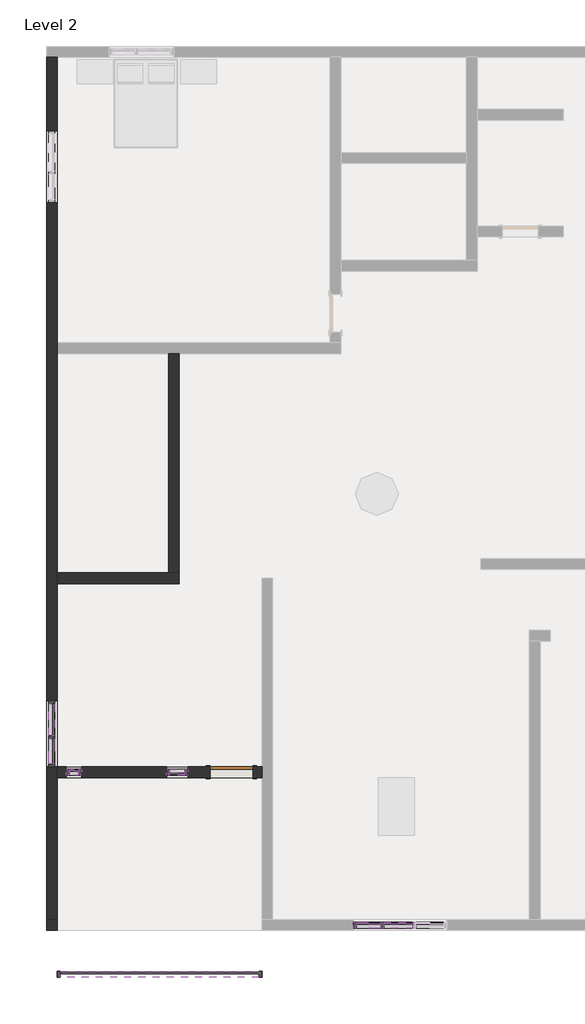
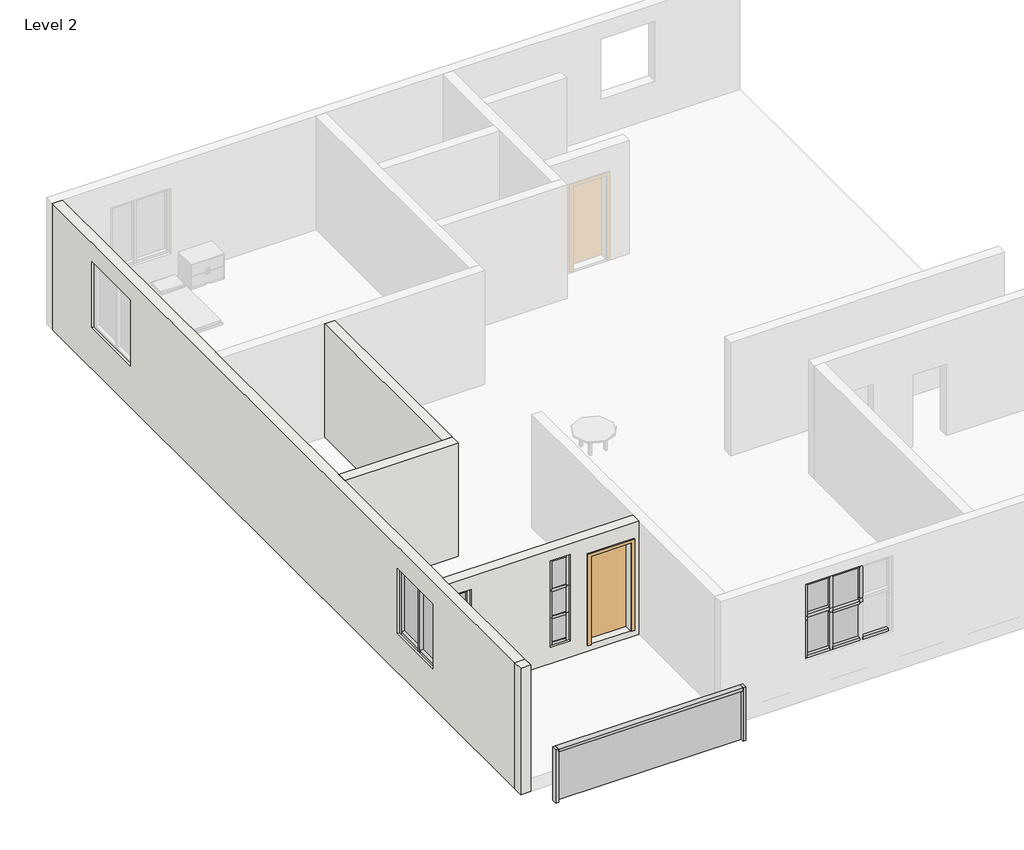
# One storey, part 1 of 3: 45 members, 13 plates, 5 walls, 1 door.
"""IFC4 building model written with IfcOpenShell, lengths in millimetres."""

from ifc_helpers import new_model, si_unit, frame, origin, place, context, project, spatial, polyline, outline, extrude, faceted_brep, transform, mapped, element, save
from components import door_0ca8825f, member_ff9f2d30, member_0c1408be, member_e5d39754, member_e31b56d3, member_3572ee78, member_a8054089, member_aa870034, member_a8964de5, member_6a93b315, member_0b7646a3, member_08dd3726, member_aaa03826, member_5b006e0e, member_fb13da3b, member_cfc5edb3, member_8ea47e38, member_081e0693, member_75a79c70, member_81de2198, member_8613ee48, member_69a5b808, member_a8c9f8c2, member_c15214c4, member_623a4a38, system_panel_glazed_ce347581, system_panel_glazed_dfb1dee4, system_panel_glazed_d46f60ed, system_panel_glazed_db16a638, system_panel_glazed_8f64e07d, system_panel_glazed_997bcd70, system_panel_glazed_706913d7, system_panel_glazed_7650606a, system_panel_glazed_1601ec89, system_panel_glazed_6c4ef35e, system_panel_glazed_6ec13f64, system_panel_glazed_f75ed1c4, system_panel_glazed_9c27a923

model = new_model("IFC4")

# Units and contexts
model_context = context("Model", 3, world=origin())
ifc_project = project(units=[si_unit("LENGTHUNIT", "METRE", prefix="MILLI")], contexts=[model_context])

# Site, building, storey
site = spatial("IfcSite", under=ifc_project)
building = spatial("IfcBuilding", under=site)
storey = spatial("IfcBuildingStorey", under=building, Name="Level 2", Elevation=3048.0)

# Door
placement = place(None, origin())
door_shape = door_0ca8825f(model_context)
element("IfcDoor", 1, ObjectType="Single-Flush : 36\" x 84\"", at=placement, inside=storey, context=model_context, shape_type="MappedRepresentation", body=[
    mapped(door_shape, transform((-15161.4702714, -8234.9383903, 3505.2), x_axis=(1.0, 0.0, 0.0), y_axis=(0.0, 1.0, 0.0), z_axis=(0.0, 0.0, 1.0))),
])

# Members
member_shape = member_ff9f2d30(model_context)
element("IfcMember", 2, ObjectType="Rectangular Mullion : 2.5\" x 5\" rectangular", at=placement, inside=storey, context=model_context, shape_type="MappedRepresentation", body=[
    mapped(member_shape, transform((-16469.5702714, -8234.9383903, 5829.1309578), x_axis=(0.0, 0.0, 1.0), y_axis=(0.0, 1.0, 0.0), z_axis=(-1.0, 0.0, 0.0))),
])
element("IfcMember", 3, ObjectType="Rectangular Mullion : 2.5\" x 5\" rectangular", at=placement, inside=storey, context=model_context, shape_type="MappedRepresentation", body=[
    mapped(member_shape, transform((-16139.3702714, -8234.9383903, 3746.1211233), x_axis=(0.0, 0.0, -1.0), y_axis=(0.0, 1.0, 0.0), z_axis=(1.0, 0.0, 0.0))),
])
member_2_shape = member_0c1408be(model_context)
element("IfcMember", 4, ObjectType="Rectangular Mullion : 2.5\" x 5\" rectangular", at=placement, inside=storey, context=model_context, shape_type="MappedRepresentation", body=[
    mapped(member_2_shape, transform((-16469.5702714, -8234.9383903, 5067.1309578), x_axis=(0.0, 0.0, 1.0), y_axis=(0.0, 1.0, 0.0), z_axis=(-1.0, 0.0, 0.0))),
])
element("IfcMember", 5, ObjectType="Rectangular Mullion : 2.5\" x 5\" rectangular", at=placement, inside=storey, context=model_context, shape_type="MappedRepresentation", body=[
    mapped(member_2_shape, transform((-16469.5702714, -8234.9383903, 4406.6260406), x_axis=(0.0, 0.0, 1.0), y_axis=(0.0, 1.0, 0.0), z_axis=(-1.0, 0.0, 0.0))),
])
member_3_shape = member_e5d39754(model_context)
element("IfcMember", 6, ObjectType="Rectangular Mullion : 2.5\" x 5\" rectangular", at=placement, inside=storey, context=model_context, shape_type="MappedRepresentation", body=[
    mapped(member_3_shape, transform((-11243.5202714, -11473.4383903, 4012.7558847), x_axis=(0.0, 0.0, -1.0), y_axis=(0.0, -1.0, 0.0), z_axis=(-1.0, 0.0, 0.0))),
])
member_4_shape = member_e31b56d3(model_context)
element("IfcMember", 7, ObjectType="Rectangular Mullion : 2.5\" x 5\" rectangular", at=placement, inside=storey, context=model_context, shape_type="MappedRepresentation", body=[
    mapped(member_4_shape, transform((-18666.6702714, -8234.9383903, 5016.6712267), x_axis=(-1.0, 0.0, 0.0), y_axis=(0.0, -1.0, 0.0), z_axis=(0.0, 0.0, 1.0))),
])
element("IfcMember", 8, ObjectType="Rectangular Mullion : 2.5\" x 5\" rectangular", at=placement, inside=storey, context=model_context, shape_type="MappedRepresentation", body=[
    mapped(member_4_shape, transform((-18666.6702714, -8234.9383903, 4376.9636561), x_axis=(-1.0, 0.0, 0.0), y_axis=(0.0, -1.0, 0.0), z_axis=(0.0, 0.0, 1.0))),
])
member_5_shape = member_3572ee78(model_context)
element("IfcMember", 9, ObjectType="Rectangular Mullion : 2.5\" x 5\" rectangular", at=placement, inside=storey, context=model_context, shape_type="MappedRepresentation", body=[
    mapped(member_5_shape, transform((-18399.9702714, -8234.9383903, 5016.6712267), x_axis=(0.0, 0.0, 1.0), y_axis=(0.0, -1.0, 0.0), z_axis=(1.0, 0.0, 0.0))),
])
element("IfcMember", 10, ObjectType="Rectangular Mullion : 2.5\" x 5\" rectangular", at=placement, inside=storey, context=model_context, shape_type="MappedRepresentation", body=[
    mapped(member_5_shape, transform((-18399.9702714, -8234.9383903, 4376.9636561), x_axis=(0.0, 0.0, 1.0), y_axis=(0.0, -1.0, 0.0), z_axis=(1.0, 0.0, 0.0))),
])
member_6_shape = member_a8054089(model_context)
element("IfcMember", 11, ObjectType="Rectangular Mullion : 2.5\" x 5\" rectangular", at=placement, inside=storey, context=model_context, shape_type="MappedRepresentation", body=[
    mapped(member_6_shape, transform((-18603.1702714, -8234.9383903, 3737.2560855), x_axis=(0.0, 0.0, -1.0), y_axis=(0.0, -1.0, 0.0), z_axis=(-1.0, 0.0, 0.0))),
])
element("IfcMember", 12, ObjectType="Rectangular Mullion : 2.5\" x 5\" rectangular", at=placement, inside=storey, context=model_context, shape_type="MappedRepresentation", body=[
    mapped(member_4_shape, transform((-18336.4702714, -8234.9383903, 4376.9636561), x_axis=(1.0, 0.0, 0.0), y_axis=(0.0, -1.0, 0.0), z_axis=(0.0, 0.0, -1.0))),
])
element("IfcMember", 13, ObjectType="Rectangular Mullion : 2.5\" x 5\" rectangular", at=placement, inside=storey, context=model_context, shape_type="MappedRepresentation", body=[
    mapped(member_4_shape, transform((-18336.4702714, -8234.9383903, 3737.2560855), x_axis=(1.0, 0.0, 0.0), y_axis=(0.0, -1.0, 0.0), z_axis=(0.0, 0.0, -1.0))),
])
element("IfcMember", 14, ObjectType="Rectangular Mullion : 2.5\" x 5\" rectangular", at=placement, inside=storey, context=model_context, shape_type="MappedRepresentation", body=[
    mapped(member_6_shape, transform((-18399.9702714, -8234.9383903, 5778.6712267), x_axis=(0.0, 0.0, 1.0), y_axis=(0.0, -1.0, 0.0), z_axis=(1.0, 0.0, 0.0))),
])
member_7_shape = member_aa870034(model_context)
element("IfcMember", 15, ObjectType="Rectangular Mullion : 2.5\" x 5\" rectangular", at=placement, inside=storey, context=model_context, shape_type="MappedRepresentation", body=[
    mapped(member_7_shape, transform((-18666.6702714, -8234.9383903, 5778.6712267), x_axis=(-1.0, 0.0, 0.0), y_axis=(0.0, -1.0, 0.0), z_axis=(0.0, 0.0, 1.0))),
])
element("IfcMember", 16, ObjectType="Rectangular Mullion : 2.5\" x 5\" rectangular", at=placement, inside=storey, context=model_context, shape_type="MappedRepresentation", body=[
    mapped(member_7_shape, transform((-16075.8702714, -8234.9383903, 5829.1309578), x_axis=(1.0, 0.0, 0.0), y_axis=(0.0, 1.0, 0.0), z_axis=(0.0, 0.0, 1.0))),
])
element("IfcMember", 17, ObjectType="Rectangular Mullion : 2.5\" x 5\" rectangular", at=placement, inside=storey, context=model_context, shape_type="MappedRepresentation", body=[
    mapped(member_7_shape, transform((-18336.4702714, -8234.9383903, 5016.6712267), x_axis=(1.0, 0.0, 0.0), y_axis=(0.0, -1.0, 0.0), z_axis=(0.0, 0.0, -1.0))),
])
element("IfcMember", 18, ObjectType="Rectangular Mullion : 2.5\" x 5\" rectangular", at=placement, inside=storey, context=model_context, shape_type="MappedRepresentation", body=[
    mapped(member_7_shape, transform((-16533.0702714, -8234.9383903, 5067.1309578), x_axis=(-1.0, 0.0, 0.0), y_axis=(0.0, 1.0, 0.0), z_axis=(0.0, 0.0, -1.0))),
])
member_8_shape = member_a8964de5(model_context)
element("IfcMember", 19, ObjectType="Rectangular Mullion : 2.5\" x 5\" rectangular", at=placement, inside=storey, context=model_context, shape_type="MappedRepresentation", body=[
    mapped(member_8_shape, transform((-16533.0702714, -8234.9383903, 4406.6260406), x_axis=(-1.0, 0.0, 0.0), y_axis=(0.0, 1.0, 0.0), z_axis=(0.0, 0.0, -1.0))),
])
element("IfcMember", 20, ObjectType="Rectangular Mullion : 2.5\" x 5\" rectangular", at=placement, inside=storey, context=model_context, shape_type="MappedRepresentation", body=[
    mapped(member_8_shape, transform((-16075.8702714, -8234.9383903, 5067.1309578), x_axis=(1.0, 0.0, 0.0), y_axis=(0.0, 1.0, 0.0), z_axis=(0.0, 0.0, 1.0))),
])
element("IfcMember", 21, ObjectType="Rectangular Mullion : 2.5\" x 5\" rectangular", at=placement, inside=storey, context=model_context, shape_type="MappedRepresentation", body=[
    mapped(member_8_shape, transform((-16533.0702714, -8234.9383903, 3746.1211233), x_axis=(-1.0, 0.0, 0.0), y_axis=(0.0, 1.0, 0.0), z_axis=(0.0, 0.0, -1.0))),
])
element("IfcMember", 22, ObjectType="Rectangular Mullion : 2.5\" x 5\" rectangular", at=placement, inside=storey, context=model_context, shape_type="MappedRepresentation", body=[
    mapped(member_8_shape, transform((-16075.8702714, -8234.9383903, 4406.6260406), x_axis=(1.0, 0.0, 0.0), y_axis=(0.0, 1.0, 0.0), z_axis=(0.0, 0.0, 1.0))),
])
member_9_shape = member_6a93b315(model_context)
element("IfcMember", 23, ObjectType="Rectangular Mullion : 2.5\" x 5\" rectangular", at=placement, inside=storey, context=model_context, shape_type="MappedRepresentation", body=[
    mapped(member_9_shape, transform((-12570.6702714, -11473.4383903, 4928.9320171), x_axis=(-1.0, 0.0, 0.0), y_axis=(0.0, -1.0, 0.0), z_axis=(0.0, 0.0, 1.0))),
])
member_10_shape = member_0b7646a3(model_context)
element("IfcMember", 24, ObjectType="Rectangular Mullion : 2.5\" x 5\" rectangular", at=placement, inside=storey, context=model_context, shape_type="MappedRepresentation", body=[
    mapped(member_10_shape, transform((-11992.8202714, -11473.4383903, 5845.1081495), x_axis=(0.0, 0.0, 1.0), y_axis=(0.0, -1.0, 0.0), z_axis=(1.0, 0.0, 0.0))),
])
element("IfcMember", 25, ObjectType="Rectangular Mullion : 2.5\" x 5\" rectangular", at=placement, inside=storey, context=model_context, shape_type="MappedRepresentation", body=[
    mapped(member_10_shape, transform((-12507.1702714, -11473.4383903, 4012.7558847), x_axis=(0.0, 0.0, -1.0), y_axis=(0.0, -1.0, 0.0), z_axis=(-1.0, 0.0, 0.0))),
])
member_11_shape = member_08dd3726(model_context)
element("IfcMember", 26, ObjectType="Rectangular Mullion : 2.5\" x 5\" rectangular", at=placement, inside=storey, context=model_context, shape_type="MappedRepresentation", body=[
    mapped(member_11_shape, transform((-11961.0702714, -11473.4383903, 5030.5320171), x_axis=(1.0, 0.0, 0.0), y_axis=(0.0, -1.0, 0.0), z_axis=(0.0, 0.0, -1.0))),
])
element("IfcMember", 27, ObjectType="Rectangular Mullion : 2.5\" x 5\" rectangular", at=placement, inside=storey, context=model_context, shape_type="MappedRepresentation", body=[
    mapped(member_11_shape, transform((-11275.2702714, -11473.4383903, 5030.5320171), x_axis=(1.0, 0.0, 0.0), y_axis=(0.0, -1.0, 0.0), z_axis=(0.0, 0.0, -1.0))),
])
member_12_shape = member_aaa03826(model_context)
element("IfcMember", 28, ObjectType="Rectangular Mullion : 2.5\" x 5\" rectangular", at=placement, inside=storey, context=model_context, shape_type="MappedRepresentation", body=[
    mapped(member_12_shape, transform((-11992.8202714, -11473.4383903, 5030.5320171), x_axis=(0.0, 0.0, 1.0), y_axis=(0.0, -1.0, 0.0), z_axis=(1.0, 0.0, 0.0))),
])
member_13_shape = member_5b006e0e(model_context)
element("IfcMember", 29, ObjectType="Rectangular Mullion : 2.5\" x 5\" rectangular", at=placement, inside=storey, context=model_context, shape_type="MappedRepresentation", body=[
    mapped(member_13_shape, transform((-12570.6702714, -11473.4383903, 5845.1081495), x_axis=(-1.0, 0.0, 0.0), y_axis=(0.0, -1.0, 0.0), z_axis=(0.0, 0.0, 1.0))),
])
member_14_shape = member_fb13da3b(model_context)
element("IfcMember", 30, ObjectType="Rectangular Mullion : 2.5\" x 5\" rectangular", at=placement, inside=storey, context=model_context, shape_type="MappedRepresentation", body=[
    mapped(member_14_shape, transform((-12570.6702714, -11473.4383903, 5030.5320171), x_axis=(-1.0, 0.0, 0.0), y_axis=(0.0, -1.0, 0.0), z_axis=(0.0, 0.0, 1.0))),
])
member_15_shape = member_cfc5edb3(model_context)
element("IfcMember", 31, ObjectType="Rectangular Mullion : 2.5\" x 5\" rectangular", at=placement, inside=storey, context=model_context, shape_type="MappedRepresentation", body=[
    mapped(member_15_shape, transform((-11961.0702714, -11473.4383903, 4928.9320171), x_axis=(1.0, 0.0, 0.0), y_axis=(0.0, -1.0, 0.0), z_axis=(0.0, 0.0, -1.0))),
])
element("IfcMember", 32, ObjectType="Rectangular Mullion : 2.5\" x 5\" rectangular", at=placement, inside=storey, context=model_context, shape_type="MappedRepresentation", body=[
    mapped(member_15_shape, transform((-11275.2702714, -11473.4383903, 4928.9320171), x_axis=(1.0, 0.0, 0.0), y_axis=(0.0, -1.0, 0.0), z_axis=(0.0, 0.0, -1.0))),
])
member_16_shape = member_8ea47e38(model_context)
element("IfcMember", 33, ObjectType="Rectangular Mullion : 2.5\" x 5\" rectangular", at=placement, inside=storey, context=model_context, shape_type="MappedRepresentation", body=[
    mapped(member_16_shape, transform((-11961.0702714, -11473.4383903, 4012.7558847), x_axis=(1.0, 0.0, 0.0), y_axis=(0.0, -1.0, 0.0), z_axis=(0.0, 0.0, -1.0))),
])
member_17_shape = member_081e0693(model_context)
element("IfcMember", 34, ObjectType="Rectangular Mullion : 2.5\" x 5\" rectangular", at=placement, inside=storey, context=model_context, shape_type="MappedRepresentation", body=[
    mapped(member_17_shape, transform((-11929.3202714, -11473.4383903, 4012.7558847), x_axis=(0.0, 0.0, -1.0), y_axis=(0.0, -1.0, 0.0), z_axis=(-1.0, 0.0, 0.0))),
])
element("IfcMember", 35, ObjectType="Rectangular Mullion : 2.5\" x 5\" rectangular", at=placement, inside=storey, context=model_context, shape_type="MappedRepresentation", body=[
    mapped(member_17_shape, transform((-11307.0202714, -11473.4383903, 5845.1081495), x_axis=(0.0, 0.0, 1.0), y_axis=(0.0, -1.0, 0.0), z_axis=(1.0, 0.0, 0.0))),
])
member_18_shape = member_75a79c70(model_context)
element("IfcMember", 36, ObjectType="Rectangular Mullion : 2.5\" x 5\" rectangular", at=placement, inside=storey, context=model_context, shape_type="MappedRepresentation", body=[
    mapped(member_18_shape, transform((-11307.0202714, -11473.4383903, 4928.9320171), x_axis=(0.0, 0.0, 1.0), y_axis=(0.0, -1.0, 0.0), z_axis=(1.0, 0.0, 0.0))),
])
member_19_shape = member_81de2198(model_context)
element("IfcMember", 37, ObjectType="Rectangular Mullion : 2.5\" x 5\" rectangular", at=placement, inside=storey, context=model_context, shape_type="MappedRepresentation", body=[
    mapped(member_19_shape, transform((-18971.4702714, -8057.1383903, 5555.3141516), x_axis=(0.0, 0.0, 1.0), y_axis=(-1.0, 0.0, 0.0), z_axis=(0.0, -1.0, 0.0))),
])
element("IfcMember", 38, ObjectType="Rectangular Mullion : 2.5\" x 5\" rectangular", at=placement, inside=storey, context=model_context, shape_type="MappedRepresentation", body=[
    mapped(member_19_shape, transform((-18971.4702714, -7517.3883903, 3979.8466642), x_axis=(0.0, 0.0, -1.0), y_axis=(-1.0, 0.0, 0.0), z_axis=(0.0, 1.0, 0.0))),
])
member_20_shape = member_8613ee48(model_context)
element("IfcMember", 39, ObjectType="Rectangular Mullion : 2.5\" x 5\" rectangular", at=placement, inside=storey, context=model_context, shape_type="MappedRepresentation", body=[
    mapped(member_20_shape, transform((-18971.4702714, -7453.8883903, 5555.3141516), x_axis=(0.0, 0.0, 1.0), y_axis=(-1.0, 0.0, 0.0), z_axis=(0.0, -1.0, 0.0))),
])
member_21_shape = member_69a5b808(model_context)
element("IfcMember", 40, ObjectType="Rectangular Mullion : 2.5\" x 5\" rectangular", at=placement, inside=storey, context=model_context, shape_type="MappedRepresentation", body=[
    mapped(member_21_shape, transform((-18971.4702714, -7485.6383903, 3979.8466642), x_axis=(0.0, -1.0, 0.0), y_axis=(-1.0, 0.0, 0.0), z_axis=(0.0, 0.0, -1.0))),
])
element("IfcMember", 41, ObjectType="Rectangular Mullion : 2.5\" x 5\" rectangular", at=placement, inside=storey, context=model_context, shape_type="MappedRepresentation", body=[
    mapped(member_20_shape, transform((-18971.4702714, -6774.4383903, 3979.8466642), x_axis=(0.0, 0.0, -1.0), y_axis=(-1.0, 0.0, 0.0), z_axis=(0.0, 1.0, 0.0))),
])
member_22_shape = member_a8c9f8c2(model_context)
element("IfcMember", 42, ObjectType="Rectangular Mullion : 2.5\" x 5\" rectangular", at=placement, inside=storey, context=model_context, shape_type="MappedRepresentation", body=[
    mapped(member_22_shape, transform((-18971.4702714, -6710.9383903, 5555.3141516), x_axis=(0.0, 1.0, 0.0), y_axis=(-1.0, 0.0, 0.0), z_axis=(0.0, 0.0, 1.0))),
])
element("IfcMember", 43, ObjectType="Rectangular Mullion : 2.5\" x 5\" rectangular", at=placement, inside=storey, context=model_context, shape_type="MappedRepresentation", body=[
    mapped(member_22_shape, transform((-18971.4702714, -8120.6383903, 3979.8466642), x_axis=(0.0, -1.0, 0.0), y_axis=(-1.0, 0.0, 0.0), z_axis=(0.0, 0.0, -1.0))),
])
member_23_shape = member_c15214c4(model_context)
element("IfcMember", 44, ObjectType="Rectangular Mullion : 2.5\" x 5\" rectangular", at=placement, inside=storey, context=model_context, shape_type="MappedRepresentation", body=[
    mapped(member_23_shape, transform((-18857.1702714, -12520.0349955, 4647.0701096), x_axis=(-1.0, 0.0, 0.0), y_axis=(0.0, -1.0, 0.0), z_axis=(0.0, 0.0, 1.0))),
])
member_24_shape = member_623a4a38(model_context)
element("IfcMember", 45, ObjectType="Rectangular Mullion : 2.5\" x 5\" rectangular", at=placement, inside=storey, context=model_context, shape_type="MappedRepresentation", body=[
    mapped(member_24_shape, transform((-14577.2702714, -12520.0349955, 4647.0701096), x_axis=(0.0, 0.0, 1.0), y_axis=(0.0, -1.0, 0.0), z_axis=(1.0, 0.0, 0.0))),
])
element("IfcMember", 46, ObjectType="Rectangular Mullion : 2.5\" x 5\" rectangular", at=placement, inside=storey, context=model_context, shape_type="MappedRepresentation", body=[
    mapped(member_23_shape, transform((-14513.7702714, -12520.0349955, 3361.4365062), x_axis=(1.0, 0.0, 0.0), y_axis=(0.0, -1.0, 0.0), z_axis=(0.0, 0.0, -1.0))),
])

# Plates
system_panel_glazed_shape = system_panel_glazed_ce347581(model_context)
element("IfcPlate", 47, ObjectType="System Panel : Glazed", at=placement, inside=storey, context=model_context, shape_type="MappedRepresentation", body=[
    mapped(system_panel_glazed_shape, transform((-18501.5702714, -8234.9383903, 3800.7560855), x_axis=(1.0, 0.0, 0.0), y_axis=(0.0, 1.0, 0.0), z_axis=(0.0, 0.0, 1.0))),
])
system_panel_glazed_2_shape = system_panel_glazed_dfb1dee4(model_context)
element("IfcPlate", 48, ObjectType="System Panel : Glazed", at=placement, inside=storey, context=model_context, shape_type="MappedRepresentation", body=[
    mapped(system_panel_glazed_2_shape, transform((-18501.5702714, -8234.9383903, 4408.7136561), x_axis=(1.0, 0.0, 0.0), y_axis=(0.0, 1.0, 0.0), z_axis=(0.0, 0.0, 1.0))),
])
system_panel_glazed_3_shape = system_panel_glazed_d46f60ed(model_context)
element("IfcPlate", 49, ObjectType="System Panel : Glazed", at=placement, inside=storey, context=model_context, shape_type="MappedRepresentation", body=[
    mapped(system_panel_glazed_3_shape, transform((-18501.5702714, -8234.9383903, 5048.4212267), x_axis=(1.0, 0.0, 0.0), y_axis=(0.0, 1.0, 0.0), z_axis=(0.0, 0.0, 1.0))),
])
system_panel_glazed_4_shape = system_panel_glazed_db16a638(model_context)
element("IfcPlate", 50, ObjectType="System Panel : Glazed", at=placement, inside=storey, context=model_context, shape_type="MappedRepresentation", body=[
    mapped(system_panel_glazed_4_shape, transform((-16304.4702714, -8234.9383903, 5098.8809578), x_axis=(-1.0, 0.0, 0.0), y_axis=(0.0, -1.0, 0.0), z_axis=(0.0, 0.0, 1.0))),
])
system_panel_glazed_5_shape = system_panel_glazed_8f64e07d(model_context)
element("IfcPlate", 51, ObjectType="System Panel : Glazed", at=placement, inside=storey, context=model_context, shape_type="MappedRepresentation", body=[
    mapped(system_panel_glazed_5_shape, transform((-16304.4702714, -8234.9383903, 4438.3760406), x_axis=(-1.0, 0.0, 0.0), y_axis=(0.0, -1.0, 0.0), z_axis=(0.0, 0.0, 1.0))),
])
system_panel_glazed_6_shape = system_panel_glazed_997bcd70(model_context)
element("IfcPlate", 52, ObjectType="System Panel : Glazed", at=placement, inside=storey, context=model_context, shape_type="MappedRepresentation", body=[
    mapped(system_panel_glazed_6_shape, transform((-16304.4702714, -8234.9383903, 3809.6211233), x_axis=(-1.0, 0.0, 0.0), y_axis=(0.0, -1.0, 0.0), z_axis=(0.0, 0.0, 1.0))),
])
system_panel_glazed_7_shape = system_panel_glazed_706913d7(model_context)
element("IfcPlate", 53, ObjectType="System Panel : Glazed", at=placement, inside=storey, context=model_context, shape_type="MappedRepresentation", body=[
    mapped(system_panel_glazed_7_shape, transform((-12249.9952714, -11473.4383903, 4076.2558847), x_axis=(1.0, 0.0, 0.0), y_axis=(0.0, 1.0, 0.0), z_axis=(0.0, 0.0, 1.0))),
])
system_panel_glazed_8_shape = system_panel_glazed_7650606a(model_context)
element("IfcPlate", 54, ObjectType="System Panel : Glazed", at=placement, inside=storey, context=model_context, shape_type="MappedRepresentation", body=[
    mapped(system_panel_glazed_8_shape, transform((-12249.9952714, -11473.4383903, 5062.2820171), x_axis=(1.0, 0.0, 0.0), y_axis=(0.0, 1.0, 0.0), z_axis=(0.0, 0.0, 1.0))),
])
system_panel_glazed_9_shape = system_panel_glazed_1601ec89(model_context)
element("IfcPlate", 55, ObjectType="System Panel : Glazed", at=placement, inside=storey, context=model_context, shape_type="MappedRepresentation", body=[
    mapped(system_panel_glazed_9_shape, transform((-11618.1702714, -11473.4383903, 4076.2558847), x_axis=(1.0, 0.0, 0.0), y_axis=(0.0, 1.0, 0.0), z_axis=(0.0, 0.0, 1.0))),
])
system_panel_glazed_10_shape = system_panel_glazed_6c4ef35e(model_context)
element("IfcPlate", 56, ObjectType="System Panel : Glazed", at=placement, inside=storey, context=model_context, shape_type="MappedRepresentation", body=[
    mapped(system_panel_glazed_10_shape, transform((-11618.1702714, -11473.4383903, 4960.6820171), x_axis=(1.0, 0.0, 0.0), y_axis=(0.0, 1.0, 0.0), z_axis=(0.0, 0.0, 1.0))),
])
system_panel_glazed_11_shape = system_panel_glazed_6ec13f64(model_context)
element("IfcPlate", 57, ObjectType="System Panel : Glazed", at=placement, inside=storey, context=model_context, shape_type="MappedRepresentation", body=[
    mapped(system_panel_glazed_11_shape, transform((-18971.4702714, -7114.1633903, 4043.3466642), x_axis=(0.0, -1.0, 0.0), y_axis=(1.0, 0.0, 0.0), z_axis=(0.0, 0.0, 1.0))),
])
system_panel_glazed_12_shape = system_panel_glazed_f75ed1c4(model_context)
element("IfcPlate", 58, ObjectType="System Panel : Glazed", at=placement, inside=storey, context=model_context, shape_type="MappedRepresentation", body=[
    mapped(system_panel_glazed_12_shape, transform((-18971.4702714, -7787.2633903, 4043.3466642), x_axis=(0.0, -1.0, 0.0), y_axis=(1.0, 0.0, 0.0), z_axis=(0.0, 0.0, 1.0))),
])
system_panel_glazed_13_shape = system_panel_glazed_9c27a923(model_context)
element("IfcPlate", 59, ObjectType="System Panel : Glazed", at=placement, inside=storey, context=model_context, shape_type="MappedRepresentation", body=[
    mapped(system_panel_glazed_13_shape, transform((-16685.4702714, -12520.0349955, 3361.4365062), x_axis=(1.0, 0.0, 0.0), y_axis=(0.0, 1.0, 0.0), z_axis=(0.0, 0.0, 1.0))),
])

# Walls
element("IfcWall", 60, ObjectType="9\"", at=placement, inside=storey, context=model_context, shape_type="Brep", body=[
    faceted_brep([(-19085.7702714, 6928.8616097, 3048.0), (-19085.7702714, -11359.1383903, 3048.0), (-19085.7702714, -11359.1383903, 6096.0), (-19085.7702714, 6928.8616097, 6096.0), (-19085.7702714, 5366.7616097, 4041.7365925), (-19085.7702714, 5366.7616097, 5636.3811186), (-19085.7702714, 3842.7616097, 5636.3811186), (-19085.7702714, 3842.7616097, 4041.7365925), (-19085.7702714, -6710.9383903, 3979.8466642), (-19085.7702714, -6710.9383903, 5555.3141516), (-19085.7702714, -8120.6383903, 5555.3141516), (-19085.7702714, -8120.6383903, 3979.8466642), (-18857.1702714, -11359.1383903, 3048.0), (-18857.1702714, -8349.2383903, 3048.0), (-18857.1702714, -8120.6383903, 3048.0), (-18857.1702714, -4234.4383903, 3048.0), (-18857.1702714, -4005.8383903, 3048.0), (-18857.1702714, 642.3616097, 3048.0), (-18857.1702714, 870.9616097, 3048.0), (-18857.1702714, 6928.8616097, 3048.0), (-18857.1702714, 6928.8616097, 6096.0), (-18857.1702714, 870.9616097, 6096.0), (-18857.1702714, 642.3616097, 6096.0), (-18857.1702714, -4005.8383903, 6096.0), (-18857.1702714, -4234.4383903, 6096.0), (-18857.1702714, -8120.6383903, 6096.0), (-18857.1702714, -8349.2383903, 6096.0), (-18857.1702714, -11359.1383903, 6096.0), (-18857.1702714, 5366.7616097, 5636.3811186), (-18857.1702714, 5366.7616097, 4041.7365925), (-18857.1702714, 3842.7616097, 4041.7365925), (-18857.1702714, 3842.7616097, 5636.3811186), (-18857.1702714, -6710.9383903, 5555.3141516), (-18857.1702714, -6710.9383903, 3979.8466642), (-18857.1702714, -8120.6383903, 3979.8466642), (-18857.1702714, -8120.6383903, 5555.3141516)], [[[0, 1, 2, 3], [4, 5, 6, 7], [8, 9, 10, 11]], [[12, 13, 14, 15, 16, 17, 18, 19, 20, 21, 22, 23, 24, 25, 26, 27], [28, 29, 30, 31], [32, 33, 34, 35]], [[1, 0, 19, 18, 17, 16, 15, 14, 13, 12]], [[3, 2, 27, 26, 25, 24, 23, 22, 21, 20]], [[0, 3, 20, 19]], [[2, 1, 12, 27]], [[28, 5, 4, 29]], [[5, 28, 31, 6]], [[6, 31, 30, 7]], [[29, 4, 7, 30]], [[8, 33, 32, 9]], [[9, 32, 35, 10]], [[10, 35, 34, 11]], [[33, 8, 11, 34]]]),
])
element("IfcWall", 61, ObjectType="9\"", at=placement, inside=storey, context=model_context, shape_type="Brep", body=[
    faceted_brep([(-18857.1702714, -8349.2383903, 3048.0), (-14513.7702714, -8349.2383903, 3048.0), (-14513.7702714, -8349.2383903, 6096.0), (-18857.1702714, -8349.2383903, 6096.0), (-18666.6702714, -8349.2383903, 3737.2560855), (-18666.6702714, -8349.2383903, 5778.6712267), (-18336.4702714, -8349.2383903, 5778.6712267), (-18336.4702714, -8349.2383903, 3737.2560855), (-15618.6702714, -8349.2383903, 3505.2), (-15618.6702714, -8349.2383903, 5638.8), (-14704.2702714, -8349.2383903, 5638.8), (-14704.2702714, -8349.2383903, 3505.2), (-16075.8702714, -8349.2383903, 5829.1309578), (-16075.8702714, -8349.2383903, 3746.1211233), (-16533.0702714, -8349.2383903, 3746.1211233), (-16533.0702714, -8349.2383903, 5829.1309578), (-14513.7702714, -8120.6383903, 3048.0), (-18857.1702714, -8120.6383903, 3048.0), (-18857.1702714, -8120.6383903, 3979.8466642), (-18857.1702714, -8120.6383903, 5555.3141516), (-18857.1702714, -8120.6383903, 6096.0), (-14513.7702714, -8120.6383903, 6096.0), (-18666.6702714, -8120.6383903, 5778.6712267), (-18666.6702714, -8120.6383903, 3737.2560855), (-18336.4702714, -8120.6383903, 3737.2560855), (-18336.4702714, -8120.6383903, 5778.6712267), (-15618.6702714, -8120.6383903, 3505.2), (-14704.2702714, -8120.6383903, 3505.2), (-14704.2702714, -8120.6383903, 5638.8), (-15618.6702714, -8120.6383903, 5638.8), (-16075.8702714, -8120.6383903, 3746.1211233), (-16075.8702714, -8120.6383903, 5829.1309578), (-16533.0702714, -8120.6383903, 5829.1309578), (-16533.0702714, -8120.6383903, 3746.1211233)], [[[0, 1, 2, 3], [4, 5, 6, 7], [8, 9, 10, 11], [12, 13, 14, 15]], [[16, 17, 18, 19, 20, 21], [22, 23, 24, 25], [26, 27, 28, 29], [30, 31, 32, 33]], [[1, 0, 17, 16]], [[3, 2, 21, 20]], [[0, 3, 20, 19, 18, 17]], [[2, 1, 16, 21]], [[22, 5, 4, 23]], [[5, 22, 25, 6]], [[6, 25, 24, 7]], [[23, 4, 7, 24]], [[27, 26, 8, 11]], [[28, 27, 11, 10]], [[29, 28, 10, 9]], [[26, 29, 9, 8]], [[30, 13, 12, 31]], [[31, 12, 15, 32]], [[32, 15, 14, 33]], [[13, 30, 33, 14]]]),
])
element("IfcWall", 62, ObjectType="9\"", at=placement, inside=storey, context=model_context, shape_type="Brep", body=[
    faceted_brep([(-18857.1702714, -4234.4383903, 3048.0), (-16266.3702714, -4234.4383903, 3048.0), (-16266.3702714, -4234.4383903, 6096.0), (-18857.1702714, -4234.4383903, 6096.0), (-18857.1702714, -4005.8383903, 3048.0), (-18857.1702714, -4005.8383903, 6096.0), (-16494.9702714, -4005.8383903, 6096.0), (-16266.3702714, -4005.8383903, 6096.0), (-16266.3702714, -4005.8383903, 3048.0), (-16494.9702714, -4005.8383903, 3048.0)], [[[0, 1, 2, 3]], [[4, 5, 6, 7, 8, 9]], [[1, 0, 4, 9, 8]], [[3, 2, 7, 6, 5]], [[0, 3, 5, 4]], [[2, 1, 8, 7]]]),
])
element("IfcWall", 63, ObjectType="9\"", at=placement, inside=storey, context=model_context, shape_type="SweptSolid", body=[
    extrude(outline(polyline([(-16266.3702714, 642.3616097), (-16266.3702714, -4005.8383903), (-16494.9702714, -4005.8383903), (-16494.9702714, 642.3616097), (-16266.3702714, 642.3616097)])), frame((0.0, 0.0, 3048.0), z_axis=(0.0, 0.0, 1.0), x_axis=(1.0, 0.0, 0.0)), (0.0, 0.0, 1.0), 3048.0),
])
element("IfcWall", 64, ObjectType="9\"", at=placement, inside=storey, context=model_context, shape_type="SweptSolid", body=[
    extrude(outline(polyline([(-19085.7702714, -11359.1383903), (-18857.1702714, -11359.1383903), (-18857.1702714, -11587.7383903), (-19085.7702714, -11587.7383903), (-19085.7702714, -11359.1383903)])), frame((0.0, 0.0, 3048.0), z_axis=(0.0, 0.0, 1.0), x_axis=(1.0, 0.0, 0.0)), (0.0, 0.0, 1.0), 3048.0),
])

save(model, "model.ifc")

# Revit data of these elements
# Type "Single-Flush : 36\" x 84\""
#   Type Mark = "1"
#   Construction Type Id = "MDOOR"
#   Assembly Code = "C1020"
#   Analytic Construction = "Metal"
#   Thickness = 0' - 2"
#   Heat Transfer Coefficient (U) = 0.651978 BTU/(h·ft²·°F)
#   Height = 7' - 0"
#   Trim Projection Ext = 0' - 1"
#   Trim Projection Int = 0' - 1"
#   Trim Width = 0' - 3"
#   Width = 3' - 0"
#   Define Thermal Properties by = 1
#   Define Thermal Properties by = 1
#   Door Material = Door - Panel
#   Frame Material = Door - Frame
#   Visual Light Transmittance = 0
#   Solar Heat Gain Coefficient = 0
#   Function = (empty or 0)
#   Wall Closure = (empty or 0)
# Type "Rectangular Mullion : 2.5\" x 5\" rectangular"
#   built-in parameter 1007304 = 0.416667 (stored number, unit not read)
#   built-in parameter 1007301 = 0.104167 (stored number, unit not read)
#   built-in parameter 1007300 = 0.104167 (stored number, unit not read)
# Type "System Panel : Glazed"
#   Construction Type Id = "GSP4R"
#   Analytic Construction = "1/8 in Pilkington single glazing"
#   Visual Light Transmittance = 0.9
#   Solar Heat Gain Coefficient = 0.86
#   Heat Transfer Coefficient (U) = 1.18115 BTU/(h·ft²·°F)
#   Define Thermal Properties by = 1
# Type "9\""
#   Assembly Code = "B2010"
#   Layers, outside or top first: 0' - 9" no material (function 1)
# Element 1 (IfcDoor, "Single-Flush : 36\" x 84\"")
#   Phase Created = New Construction
#   Materials on its faces: "Door - Frame", "Door - Panel"
# Elements 2, 3, 4, 5, 6, 7, 8, 9, 10, 11, 12, 13, 14, 15, 16, 17, 18, 19, 20, 21, 22, 23, 24, 25, 26, 27, 28, 29, 30, 31, 32, 33, 34, 35, 36, 37, 38, 39, 40, 41, 42, 43, 44, 45, 46 (IfcMember, "Rectangular Mullion : 2.5\" x 5\" rectangular")
#   Phase Created = New Construction
#   Materials on its faces: "Aluminum"
# Elements 47, 48, 49, 50, 51, 52, 53, 54, 55, 56, 57, 58, 59 (IfcPlate, "System Panel : Glazed")
#   Phase Created = New Construction
#   Materials on its faces: "Glass"
# Elements 60, 61, 62, 63, 64 (IfcWall, "9\"")
#   Top Offset = 0' - 0"
#   Base Offset = 0' - 0"
#   Unconnected Height = 10' - 0"
#   wall height = 10' - 0"
#   Phase Created = New Construction
#   Base Constraint = Level 2
#   Materials on its faces: "Default Wall"
# Materials
#   "Door - Panel": class "Wood", colour RGB 210 159 95, transparency 0, Cost = 0
#   "Door - Frame": colour RGB 118 70 51, transparency 0, Cost = 0
#   "Aluminum": class "Metal", colour RGB 247 247 247, transparency 0, Description = "Aluminum 6061", Cost = 0
#   "Glass": class "Glass", colour RGB 0 128 192, transparency 0.75, Description = "Soda Lime Glass", Cost = 0
#   "Default Wall": colour RGB 128 128 128, transparency 0, Cost = 0
